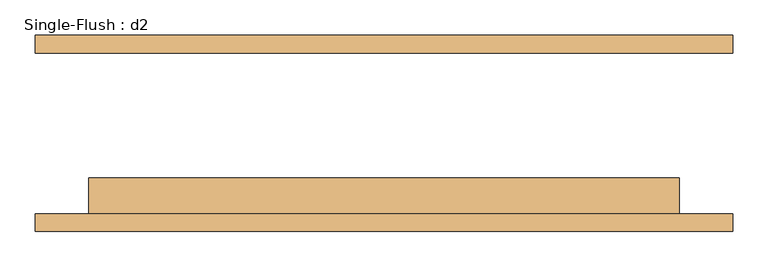
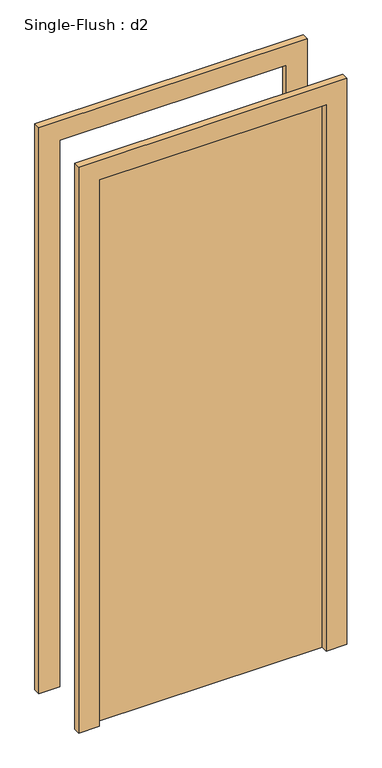
"""IFC4 building model written with IfcOpenShell, lengths in millimetres: door geometry, Single-Flush : d2."""

from ifc_helpers import new_model, si_unit, frame, origin, origin_with_axes, place, context, project, spatial, polyline, outline, extrude, source, transform, mapped, element, save


def single_flush_d2_53d9c022(model_context):
    return source(origin(), model_context, "Body", "SweptSolid", [
        extrude(outline(polyline([(2209.8, -495.3), (0.0, -495.3), (0.0, -419.1), (2133.6, -419.1), (2133.6, 419.1), (0.0, 419.1), (0.0, 495.3), (2209.8, 495.3), (2209.8, -495.3)])), frame((0.0, -139.7, 0.0), z_axis=(0.0, 1.0, 0.0), x_axis=(0.0, 0.0, 1.0)), (0.0, 0.0, 1.0), 25.4),
        extrude(outline(polyline([(2209.8, 495.3), (2209.8, -495.3), (0.0, -495.3), (0.0, -419.1), (2133.6, -419.1), (2133.6, 419.1), (0.0, 419.1), (0.0, 495.3), (2209.8, 495.3)])), frame((0.0, 114.3, 0.0), z_axis=(0.0, 1.0, 0.0), x_axis=(0.0, 0.0, 1.0)), (0.0, 0.0, 1.0), 25.4),
        extrude(outline(polyline([(419.1, -63.5), (419.1, -114.3), (-419.1, -114.3), (-419.1, -63.5), (419.1, -63.5)])), origin_with_axes(), (0.0, 0.0, 1.0), 2133.6),
    ])


if __name__ == "__main__":
    model = new_model("IFC4")
    model_context = context("Model", 3, world=origin())
    ifc_project = project(units=[si_unit("LENGTHUNIT", "METRE", prefix="MILLI")], contexts=[model_context])
    site = spatial("IfcSite", under=ifc_project)
    building = spatial("IfcBuilding", under=site)
    placement = place(None, origin())
    single_flush_d2_shape = single_flush_d2_53d9c022(model_context)
    element("IfcDoor", 1, ObjectType="Single-Flush : d2", at=placement, inside=building, context=model_context, shape_type="MappedRepresentation", body=[
        mapped(single_flush_d2_shape, transform((0.0, 0.0, 0.0), x_axis=(1.0, 0.0, 0.0), y_axis=(0.0, 1.0, 0.0), z_axis=(0.0, 0.0, 1.0))),
    ])
    save(model, "model.ifc")

# Revit data of these elements
# Type "Single-Flush : d2"
#   Type Mark = "9"
#   Construction Type Id = "MDOOR"
#   Assembly Code = "C1020"
#   Analytic Construction = "Metal"
#   Thickness = 0' - 2"
#   Heat Transfer Coefficient (U) = 0.651978 BTU/(h·ft²·°F)
#   Height = 7' - 0"
#   Trim Projection Ext = 0' - 1"
#   Trim Projection Int = 0' - 1"
#   Trim Width = 0' - 3"
#   Width = 2' - 9"
#   Define Thermal Properties by = 1
#   Door Material = Door - Panel
#   Frame Material = Door - Frame
#   Visual Light Transmittance = 0
#   Solar Heat Gain Coefficient = 0
#   Function = (empty or 0)
#   Wall Closure = (empty or 0)
# Element 1 (IfcDoor, "Single-Flush : d2")
#   Materials on its faces: "Door - Frame", "Door - Panel"
# Materials
#   "Door - Panel": class "Wood", colour RGB 210 159 95, transparency 0, Cost = 0
#   "Door - Frame": colour RGB 118 70 51, transparency 0, Cost = 0
